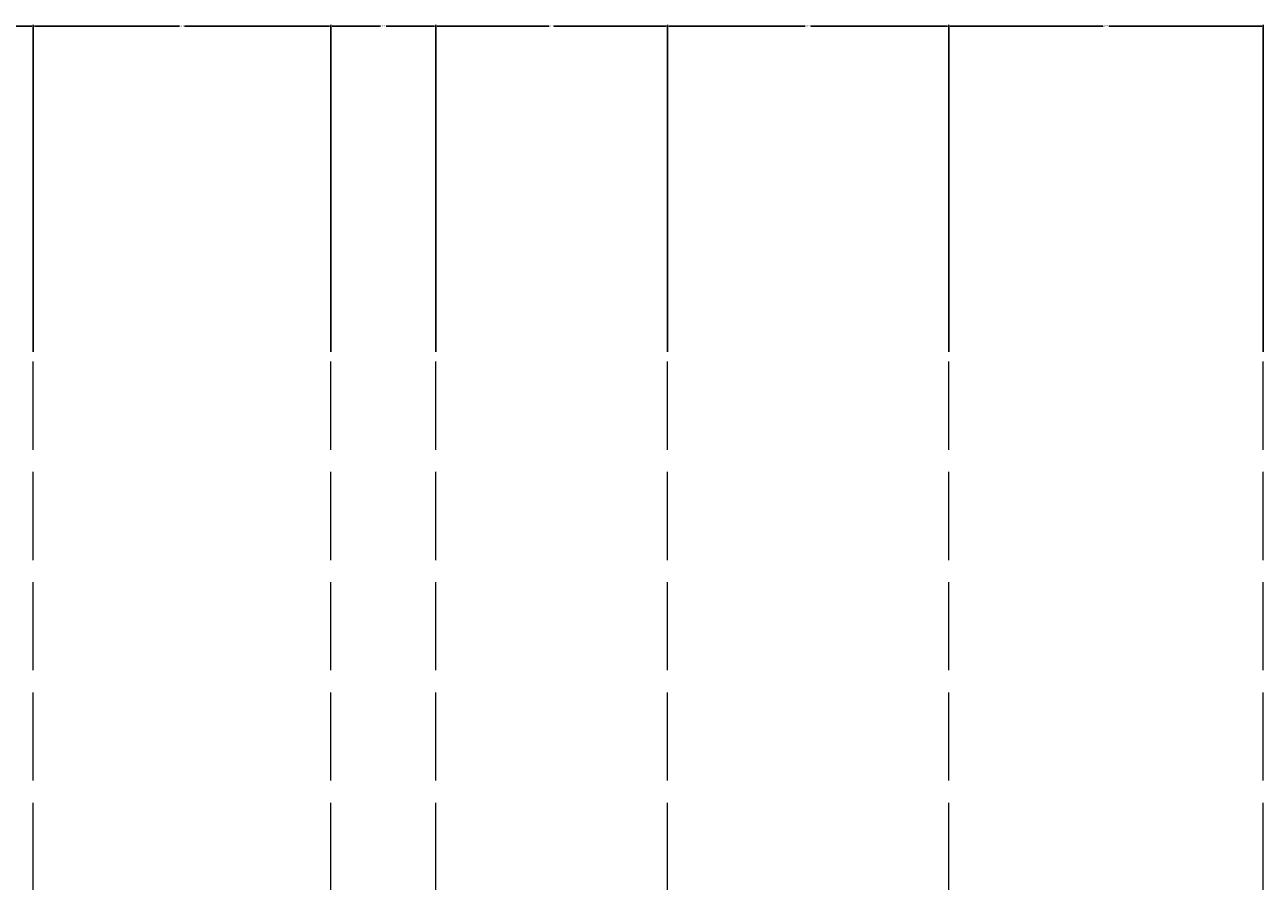
# Model space of a CAD drawing. Units: inches. Extents: x 1159 to 4240, y 1112 to 2085.
# Tile 10 of 13: x 1535 to 1704, y 1968 to 2085. Entities that reach past the tile are written whole.
import ezdxf

# ---------------------------------------------------------------- set-up
doc = ezdxf.new("R2010")
doc.units = ezdxf.units.IN
doc.linetypes.add('ACAD_ISO02W100', pattern=[15, 12, -3])
doc.layers.add('A-ANNO-DIMS', color=2, linetype='Continuous', lineweight=18)
doc.layers.add('A-GRID', color=8, linetype='ACAD_ISO02W100', lineweight=13)
doc.styles.get("Standard").update_dxf_attribs({"font": 'arial.ttf'})
doc.dimstyles.get("Standard").update_dxf_attribs({"dimtxt": 0.18, "dimasz": 0.18, "dimexe": 0.18, "dimexo": 0.0625, "dimgap": 0.09, "dimtad": 0, "dimtih": 1, "dimtoh": 1, "dimdec": 4, "dimzin": 0, "dimdsep": 46, "dimtxsty": 'Standard', "dimcen": 0.09, "dimadec": 0, "dimazin": 0, "dimtfac": 1, "dimtdec": 4, "dimtofl": 0, "dimtmove": 0, "dimatfit": 3, "dimfxl": 1, "dimtolj": 1, "dimtzin": 0, "dimarcsym": 0})

# ---------------------------------------------------------------- blocks, each defined once
blk = doc.blocks.new('HOUSE-35x60-SETTING-OUT-GRID')
for p, q in [((333.07, 0), (333.07, 883.25)), ((373.57, 0), (373.57, 883.25)), ((387.82, 0), (387.82, 883.25)), ((419.32, 0), (419.32, 883.25)), ((457.57, 0), (457.57, 883.25)), ((500.32, 0), (500.32, 883.25))]:
    blk.add_line(p, q)
blk = doc.blocks.new('*D31')
at = {"layer": 'A-ANNO-DIMS', "color": 0, "lineweight": -2, "transparency": 16777216}
for p, q in [((1459.88, 2040.27), (1459.88, 2084.73)), ((1460.06, 2084.55), (1497.8, 2084.55)), ((1536.2, 2084.55), (1498.45, 2084.55)), ((1536.38, 2040.27), (1536.38, 2084.73))]:
    blk.add_line(p, q, dxfattribs=at)
at = {"layer": 'A-ANNO-DIMS', "color": 0, "lineweight": 100, "transparency": 16777216}
for points in [[(1460.06, 2084.58), (1460.06, 2084.52), (1459.88, 2084.55)], [(1536.2, 2084.58), (1536.2, 2084.52), (1536.38, 2084.55)]]:
    blk.add_solid(points, dxfattribs=at)
at = {"layer": 'Defpoints', "color": 0, "lineweight": 100, "transparency": 16777216}
for p in [(1536.38, 2084.55), (1459.88, 2040.2), (1536.38, 2040.2)]:
    blk.add_point(p, dxfattribs=at)
at = {"layer": 'A-ANNO-DIMS', "color": 0, "transparency": 16777216, "insert": (1498.13, 2084.55), "char_height": 0.18, "attachment_point": 5}
blk.add_mtext('\\A1;76.5', dxfattribs=at)
blk = doc.blocks.new('*D32')
at = {"layer": 'A-ANNO-DIMS', "color": 0, "lineweight": -2, "transparency": 16777216}
for p, q in [((1536.38, 2040.27), (1536.38, 2084.73)), ((1536.56, 2084.55), (1556.3, 2084.55)), ((1576.7, 2084.55), (1556.95, 2084.55)), ((1576.88, 2040.27), (1576.88, 2084.73))]:
    blk.add_line(p, q, dxfattribs=at)
at = {"layer": 'A-ANNO-DIMS', "color": 0, "lineweight": 100, "transparency": 16777216}
for points in [[(1536.56, 2084.58), (1536.56, 2084.52), (1536.38, 2084.55)], [(1576.7, 2084.58), (1576.7, 2084.52), (1576.88, 2084.55)]]:
    blk.add_solid(points, dxfattribs=at)
at = {"layer": 'Defpoints', "color": 0, "lineweight": 100, "transparency": 16777216}
for p in [(1576.88, 2084.55), (1536.38, 2040.2), (1576.88, 2040.2)]:
    blk.add_point(p, dxfattribs=at)
at = {"layer": 'A-ANNO-DIMS', "color": 0, "transparency": 16777216, "insert": (1556.63, 2084.55), "char_height": 0.18, "attachment_point": 5}
blk.add_mtext('\\A1;40.5', dxfattribs=at)
blk = doc.blocks.new('*D33')
at = {"layer": 'A-ANNO-DIMS', "color": 0, "lineweight": -2, "transparency": 16777216}
for p, q in [((1576.88, 2040.27), (1576.88, 2084.73)), ((1577.06, 2084.55), (1583.61, 2084.55)), ((1590.95, 2084.55), (1584.39, 2084.55)), ((1591.13, 2040.27), (1591.13, 2084.73))]:
    blk.add_line(p, q, dxfattribs=at)
at = {"layer": 'A-ANNO-DIMS', "color": 0, "lineweight": 100, "transparency": 16777216}
for points in [[(1577.06, 2084.58), (1577.06, 2084.52), (1576.88, 2084.55)], [(1590.95, 2084.58), (1590.95, 2084.52), (1591.13, 2084.55)]]:
    blk.add_solid(points, dxfattribs=at)
at = {"layer": 'Defpoints', "color": 0, "lineweight": 100, "transparency": 16777216}
for p in [(1591.13, 2084.55), (1576.88, 2040.2), (1591.13, 2040.2)]:
    blk.add_point(p, dxfattribs=at)
at = {"layer": 'A-ANNO-DIMS', "color": 0, "transparency": 16777216, "insert": (1584, 2084.55), "char_height": 0.18, "attachment_point": 5}
blk.add_mtext('\\A1;14.25', dxfattribs=at)
blk = doc.blocks.new('*D34')
at = {"layer": 'A-ANNO-DIMS', "color": 0, "lineweight": -2, "transparency": 16777216}
for p, q in [((1591.13, 2040.27), (1591.13, 2084.73)), ((1591.31, 2084.55), (1606.55, 2084.55)), ((1622.45, 2084.55), (1607.2, 2084.55)), ((1622.63, 2040.27), (1622.63, 2084.73))]:
    blk.add_line(p, q, dxfattribs=at)
at = {"layer": 'A-ANNO-DIMS', "color": 0, "lineweight": 100, "transparency": 16777216}
for points in [[(1591.31, 2084.58), (1591.31, 2084.52), (1591.13, 2084.55)], [(1622.45, 2084.58), (1622.45, 2084.52), (1622.63, 2084.55)]]:
    blk.add_solid(points, dxfattribs=at)
at = {"layer": 'Defpoints', "color": 0, "lineweight": 100, "transparency": 16777216}
for p in [(1622.63, 2084.55), (1591.13, 2040.2), (1622.63, 2040.2)]:
    blk.add_point(p, dxfattribs=at)
at = {"layer": 'A-ANNO-DIMS', "color": 0, "transparency": 16777216, "insert": (1606.88, 2084.55), "char_height": 0.18, "attachment_point": 5}
blk.add_mtext('\\A1;31.5', dxfattribs=at)
blk = doc.blocks.new('*D35')
at = {"layer": 'A-ANNO-DIMS', "color": 0, "lineweight": -2, "transparency": 16777216}
for p, q in [((1622.63, 2040.27), (1622.63, 2084.73)), ((1622.81, 2084.55), (1641.36, 2084.55)), ((1660.7, 2084.55), (1642.14, 2084.55)), ((1660.88, 2040.27), (1660.88, 2084.73))]:
    blk.add_line(p, q, dxfattribs=at)
at = {"layer": 'A-ANNO-DIMS', "color": 0, "lineweight": 100, "transparency": 16777216}
for points in [[(1622.81, 2084.58), (1622.81, 2084.52), (1622.63, 2084.55)], [(1660.7, 2084.58), (1660.7, 2084.52), (1660.88, 2084.55)]]:
    blk.add_solid(points, dxfattribs=at)
at = {"layer": 'Defpoints', "color": 0, "lineweight": 100, "transparency": 16777216}
for p in [(1660.88, 2084.55), (1622.63, 2040.2), (1660.88, 2040.2)]:
    blk.add_point(p, dxfattribs=at)
at = {"layer": 'A-ANNO-DIMS', "color": 0, "transparency": 16777216, "insert": (1641.75, 2084.55), "char_height": 0.18, "attachment_point": 5}
blk.add_mtext('\\A1;38.25', dxfattribs=at)
blk = doc.blocks.new('*D36')
at = {"layer": 'A-ANNO-DIMS', "color": 0, "lineweight": -2, "transparency": 16777216}
for p, q in [((1660.88, 2040.27), (1660.88, 2084.73)), ((1661.06, 2084.55), (1681.85, 2084.55)), ((1703.45, 2084.55), (1682.65, 2084.55)), ((1703.63, 2040.27), (1703.63, 2084.73))]:
    blk.add_line(p, q, dxfattribs=at)
at = {"layer": 'A-ANNO-DIMS', "color": 0, "lineweight": 100, "transparency": 16777216}
for points in [[(1661.06, 2084.58), (1661.06, 2084.52), (1660.88, 2084.55)], [(1703.45, 2084.58), (1703.45, 2084.52), (1703.63, 2084.55)]]:
    blk.add_solid(points, dxfattribs=at)
at = {"layer": 'Defpoints', "color": 0, "lineweight": 100, "transparency": 16777216}
for p in [(1703.63, 2084.55), (1660.88, 2040.2), (1703.63, 2040.2)]:
    blk.add_point(p, dxfattribs=at)
at = {"layer": 'A-ANNO-DIMS', "color": 0, "transparency": 16777216, "insert": (1682.25, 2084.55), "char_height": 0.18, "attachment_point": 5}
blk.add_mtext('\\A1;42.75', dxfattribs=at)

msp = doc.modelspace()

# ---------------------------------------------------------------- block references
at = {"layer": 'A-GRID'}
msp.add_blockref('HOUSE-35x60-SETTING-OUT-GRID', (1203.31, 1156.954), dxfattribs=at)

# ---------------------------------------------------------------- dimensions: what is measured, and where the dimension line sits
at = {"layer": 'A-ANNO-DIMS'}
for base, p1, p2, override, picture, middle in [((1536.375, 2084.554), (1459.875, 2040.204), (1536.375, 2040.204), {"dimdec": 1, "dimlfac": 1, "dimrnd": 0, "dimzin": 0, "dimdsep": 46, "dimlunit": 2}, '*D31', (1498.125, 2084.554)), ((1576.875, 2084.554), (1536.375, 2040.204), (1576.875, 2040.204), {"dimdec": 1, "dimlfac": 1, "dimrnd": 0, "dimzin": 0, "dimdsep": 46, "dimlunit": 2}, '*D32', (1556.625, 2084.554)), ((1591.126, 2084.554), (1576.875, 2040.204), (1591.126, 2040.204), {"dimdec": 2, "dimlfac": 1, "dimrnd": 0, "dimzin": 0, "dimdsep": 46, "dimlunit": 2}, '*D33', (1584.001, 2084.554)), ((1622.625, 2084.554), (1591.126, 2040.204), (1622.625, 2040.204), {"dimdec": 1, "dimlfac": 1, "dimrnd": 0, "dimzin": 0, "dimdsep": 46, "dimlunit": 2}, '*D34', (1606.876, 2084.554)), ((1660.875, 2084.554), (1622.625, 2040.204), (1660.875, 2040.204), {"dimdec": 2, "dimlfac": 1, "dimrnd": 0, "dimzin": 0, "dimdsep": 46, "dimlunit": 2}, '*D35', (1641.75, 2084.554)), ((1703.625, 2084.554), (1660.875, 2040.204), (1703.625, 2040.204), {"dimdec": 2, "dimlfac": 1, "dimrnd": 0, "dimzin": 0, "dimdsep": 46, "dimlunit": 2}, '*D36', (1682.25, 2084.554))]:
    dim = msp.add_linear_dim(base=base, p1=p1, p2=p2, dimstyle='Standard', override=override, dxfattribs=at)
    dim.commit()
    dim.dimension.update_dxf_attribs({"geometry": picture, "text_midpoint": middle})

doc.saveas('drawing.dxf')
